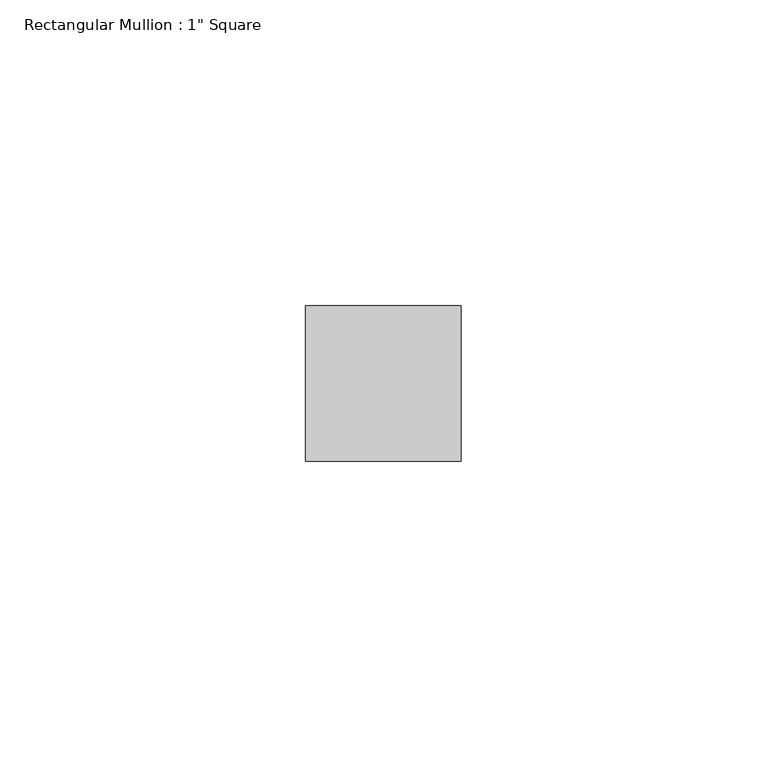
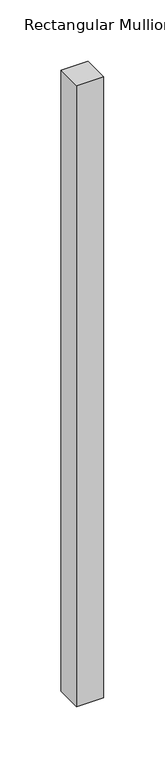
"""IFC4 building model written with IfcOpenShell, lengths in millimetres: member geometry."""

from ifc_helpers import new_model, si_unit, frame, origin, place, context, project, spatial, polyline, outline, extrude, source, transform, mapped, element, save


def member_3995c9cc(model_context):
    return source(origin(), model_context, "Body", "SweptSolid", [
        extrude(outline(polyline([(0.0, 12.7), (0.0, -12.7), (-25.4, -12.7), (-25.4, 12.7), (0.0, 12.7)])), frame((0.0, 0.0, -618.0666667), z_axis=(0.0, 0.0, 1.0), x_axis=(1.0, 0.0, 0.0)), (0.0, 0.0, 1.0), 618.0666667),
    ])


if __name__ == "__main__":
    model = new_model("IFC4")
    model_context = context("Model", 3, world=origin())
    ifc_project = project(units=[si_unit("LENGTHUNIT", "METRE", prefix="MILLI")], contexts=[model_context])
    site = spatial("IfcSite", under=ifc_project)
    building = spatial("IfcBuilding", under=site)
    placement = place(None, origin())
    member_shape = member_3995c9cc(model_context)
    element("IfcMember", 1, ObjectType="Rectangular Mullion : 1\" Square", at=placement, inside=building, context=model_context, shape_type="MappedRepresentation", body=[
        mapped(member_shape, transform((0.0, 0.0, 0.0), x_axis=(1.0, 0.0, 0.0), y_axis=(0.0, 1.0, 0.0), z_axis=(0.0, 0.0, 1.0))),
    ])
    save(model, "model.ifc")

# Revit data of these elements
# Type "Rectangular Mullion : 1\" Square"
#   built-in parameter 1007304 = 0.0833333 (stored number, unit not read)
#   built-in parameter 1007301 = 0.0416667 (stored number, unit not read)
#   built-in parameter 1007300 = 0.0416667 (stored number, unit not read)
# Element 1 (IfcMember, "Rectangular Mullion : 1\" Square")
#   Materials on its faces: "Aluminum"
# Materials
#   "Aluminum": class "Metal", colour RGB 247 247 247, transparency 0, Description = "Aluminum 6061", Cost = 0
